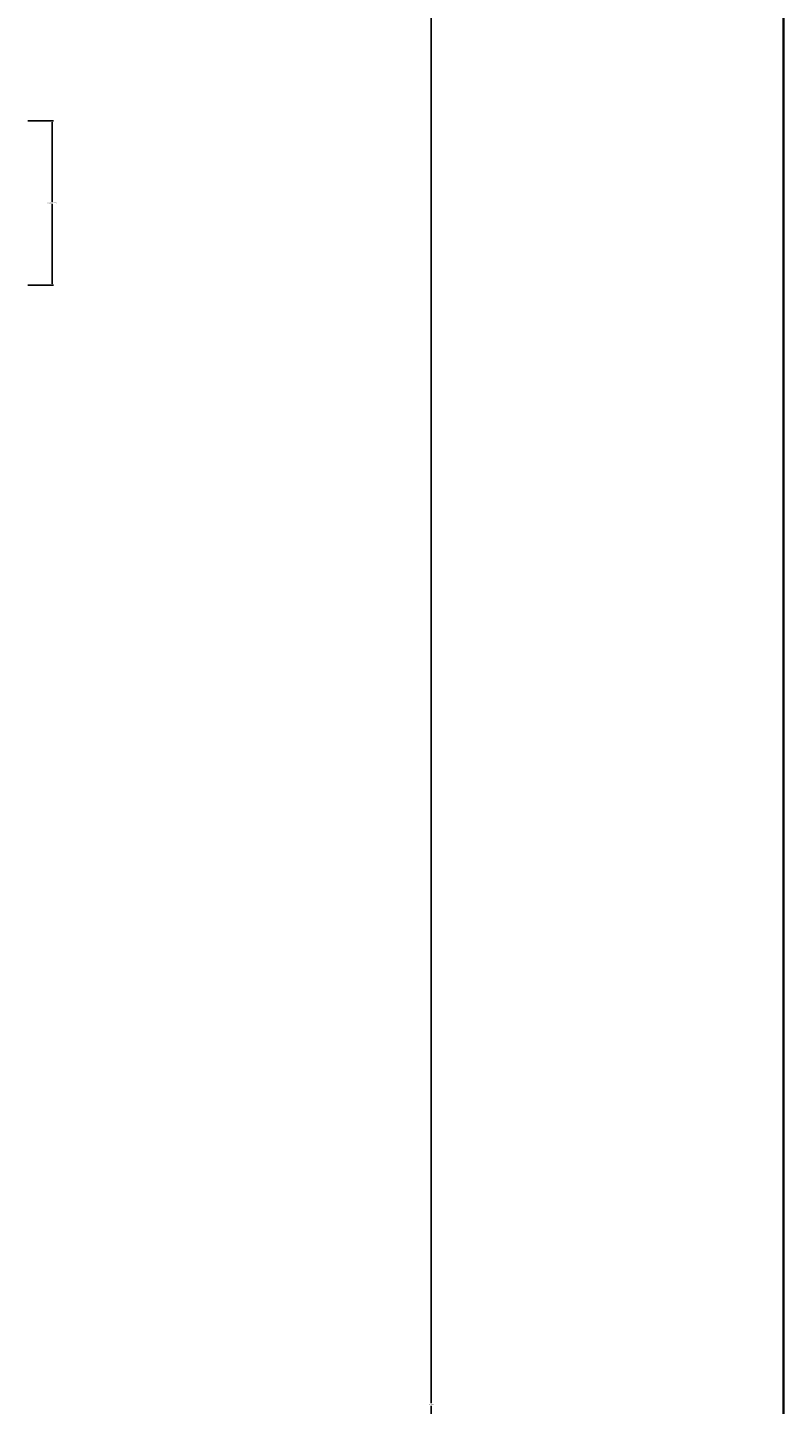
# Model space of a CAD drawing. Units: inches. Extents: x 1962 to 2771, y 1245 to 2660.
# Tile 84 of 114: x 2661 to 2771, y 1979 to 2180. Entities that reach past the tile are written whole.
import ezdxf

# ---------------------------------------------------------------- set-up
doc = ezdxf.new("R2010")
doc.units = ezdxf.units.IN
doc.layers.add('A-ANNO-DIMS', color=2, linetype='Continuous', lineweight=18)
doc.layers.add('A-ANNO-TTLB', color=7, linetype='Continuous', lineweight=35)
doc.styles.get("Standard").update_dxf_attribs({"font": 'arial.ttf'})
doc.dimstyles.get("Standard").update_dxf_attribs({"dimtxt": 0.18, "dimasz": 0.18, "dimexe": 0.18, "dimexo": 0.0625, "dimgap": 0.09, "dimtad": 0, "dimtih": 1, "dimtoh": 1, "dimdec": 4, "dimzin": 0, "dimdsep": 46, "dimtxsty": 'Standard', "dimcen": 0.09, "dimadec": 0, "dimazin": 0, "dimtfac": 1, "dimtdec": 4, "dimtofl": 0, "dimtmove": 0, "dimatfit": 3, "dimfxl": 1, "dimtolj": 1, "dimtzin": 0, "dimarcsym": 0})

# ---------------------------------------------------------------- blocks, each defined once
blk = doc.blocks.new('*D20')
at = {"layer": 'A-ANNO-DIMS', "color": 0, "lineweight": -2, "transparency": 16777216}
for p, q in [((2660.87, 2166.48), (2664.59, 2166.48)), ((2664.41, 2166.3), (2664.41, 2154.66)), ((2664.41, 2142.66), (2664.41, 2154.3)), ((2660.87, 2142.48), (2664.59, 2142.48))]:
    blk.add_line(p, q, dxfattribs=at)
at = {"layer": 'A-ANNO-DIMS', "color": 0, "transparency": 16777216}
for points in [[(2664.38, 2166.3), (2664.44, 2166.3), (2664.41, 2166.48)], [(2664.38, 2142.66), (2664.44, 2142.66), (2664.41, 2142.48)]]:
    blk.add_solid(points, dxfattribs=at)
at = {"layer": 'Defpoints', "color": 0, "transparency": 16777216}
for p in [(2660.81, 2166.48), (2664.41, 2166.48), (2660.81, 2142.48)]:
    blk.add_point(p, dxfattribs=at)
at = {"layer": 'A-ANNO-DIMS', "color": 0, "transparency": 16777216, "insert": (2664.41, 2154.48), "char_height": 0.18, "attachment_point": 5}
blk.add_mtext('\\A1;W1B 24 TYP.', dxfattribs=at)
blk = doc.blocks.new('*D40')
at = {"layer": 'A-ANNO-DIMS', "color": 0, "lineweight": -2, "transparency": 16777216}
for p, q in [((2072.02, 2033.91), (2072.02, 2583.47)), ((2072.2, 2583.29), (2366.02, 2583.29)), ((2660.63, 2583.29), (2366.81, 2583.29)), ((2660.81, 2524.41), (2660.81, 2583.47))]:
    blk.add_line(p, q, dxfattribs=at)
at = {"layer": 'A-ANNO-DIMS', "color": 0, "transparency": 16777216}
for points in [[(2072.2, 2583.32), (2072.2, 2583.26), (2072.02, 2583.29)], [(2660.63, 2583.32), (2660.63, 2583.26), (2660.81, 2583.29)]]:
    blk.add_solid(points, dxfattribs=at)
at = {"layer": 'Defpoints', "color": 0, "transparency": 16777216}
for p in [(2660.81, 2583.29), (2660.81, 2524.34), (2072.02, 2033.84)]:
    blk.add_point(p, dxfattribs=at)
at = {"layer": 'A-ANNO-DIMS', "color": 0, "transparency": 16777216, "insert": (2366.41, 2583.29), "char_height": 0.18, "attachment_point": 5}
blk.add_mtext('\\A1;588.8', dxfattribs=at)
blk = doc.blocks.new('*D42')
at = {"layer": 'A-ANNO-DIMS', "color": 0, "lineweight": -2, "transparency": 16777216}
for p, q in [((2660.87, 2524.34), (2719.94, 2524.34)), ((2719.76, 2524.16), (2719.76, 1979.28)), ((2719.76, 1434.02), (2719.76, 1978.91)), ((2660.87, 1433.84), (2719.94, 1433.84))]:
    blk.add_line(p, q, dxfattribs=at)
at = {"layer": 'A-ANNO-DIMS', "color": 0, "transparency": 16777216}
for points in [[(2719.73, 2524.16), (2719.79, 2524.16), (2719.76, 2524.34)], [(2719.73, 1434.02), (2719.79, 1434.02), (2719.76, 1433.84)]]:
    blk.add_solid(points, dxfattribs=at)
at = {"layer": 'Defpoints', "color": 0, "transparency": 16777216}
for p in [(2660.81, 2524.34), (2719.76, 2524.34), (2660.81, 1433.84)]:
    blk.add_point(p, dxfattribs=at)
at = {"layer": 'A-ANNO-DIMS', "color": 0, "transparency": 16777216, "insert": (2719.76, 1979.09), "char_height": 0.18, "attachment_point": 5}
blk.add_mtext('\\A1;1090.5', dxfattribs=at)

msp = doc.modelspace()

# ---------------------------------------------------------------- linework, layer by layer
at = {"layer": 'A-ANNO-TTLB'}
msp.add_lwpolyline([(1961.7365, 2660.2579), (2771.213, 2660.2579), (2771.213, 1244.5817), (1961.7365, 1244.5817)], close=True, dxfattribs=at)

# ---------------------------------------------------------------- dimensions: what is measured, and where the dimension line sits
at = {"layer": 'A-ANNO-DIMS'}
dim = msp.add_linear_dim(base=(2660.8074, 2583.2937), p1=(2072.0204, 2033.8437), p2=(2660.8074, 2524.3437), dimstyle='Standard', override={"dimdec": 1, "dimlfac": 1, "dimrnd": 0, "dimzin": 0, "dimdsep": 46, "dimlunit": 2}, dxfattribs=at)
dim.commit()
dim.dimension.update_dxf_attribs({"geometry": '*D40', "text_midpoint": (2366.4139, 2583.2937)})
dim = msp.add_linear_dim(base=(2719.7574, 2524.3437), p1=(2660.8074, 1433.8437), p2=(2660.8074, 2524.3437), angle=90, dimstyle='Standard', override={"dimdec": 1, "dimlfac": 1, "dimrnd": 0, "dimzin": 0, "dimdsep": 46, "dimlunit": 2}, dxfattribs=at)
dim.commit()
dim.dimension.update_dxf_attribs({"geometry": '*D42', "text_midpoint": (2719.7574, 1979.0937)})
dim = msp.add_linear_dim(base=(2664.4074, 2166.4846), p1=(2660.8074, 2142.4846), p2=(2660.8074, 2166.4846), angle=90, text='W1B <> TYP.', dimstyle='Standard', override={"dimdec": 0, "dimlfac": 1, "dimrnd": 0, "dimzin": 0, "dimdsep": 46, "dimlunit": 2}, dxfattribs=at)
dim.commit()
dim.dimension.update_dxf_attribs({"geometry": '*D20', "text_midpoint": (2664.4074, 2154.4846)})

doc.saveas('drawing.dxf')
